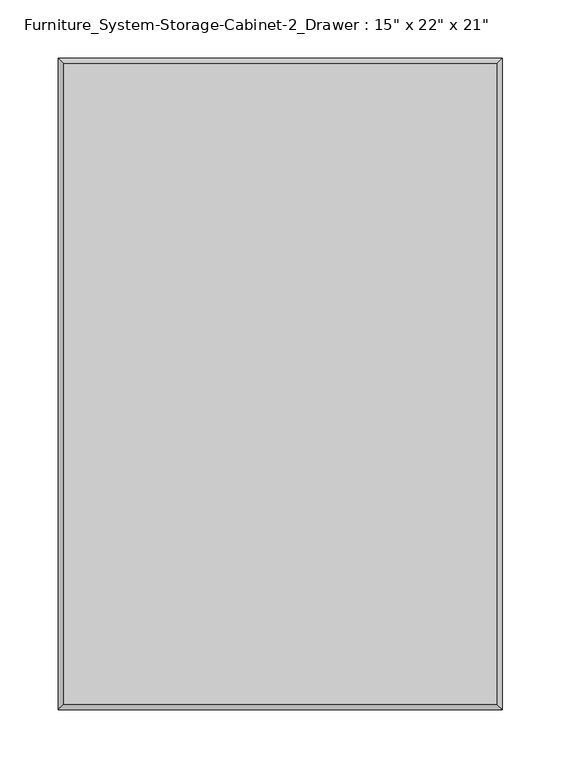
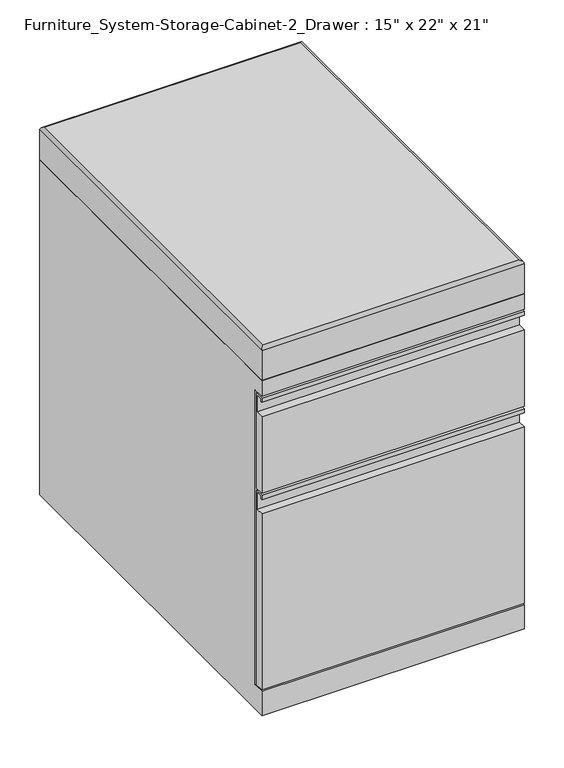
"""IFC4 building model written with IfcOpenShell, lengths in millimetres: furniture geometry."""

from ifc_helpers import new_model, si_unit, frame, origin, place, context, project, spatial, polyline, ellipse_curve, outline, extrude, source, transform, mapped, element, save
from ifc_brep_helpers import plane_surface, cylinder_surface, advanced_brep


def furniture_b20b6c06(model_context):
    return source(origin(), model_context, "Body", "SolidModel", [
        extrude(outline(polyline([(0.0, 360.3625), (0.0, 478.2451302), (11.8998876, 478.2451302), (11.8998876, 504.8884893), (1.5239879, 504.8884893), (1.5239879, 500.0625121), (0.0, 500.0625121), (0.0, 506.4124879), (13.4873883, 506.4124879), (13.4873883, 360.3625), (0.0, 360.3625)])), frame((-190.5, 0.0, 0.0), z_axis=(1.0, 0.0, 0.0), x_axis=(0.0, 1.0, 0.0)), (0.0, 0.0, 1.0), 381.0),
        extrude(outline(polyline([(0.0, 58.7374985), (0.0, 329.0201544), (11.9293774, 329.0201544), (11.9293774, 355.6635136), (1.5239879, 355.6635136), (1.5239879, 350.8375), (0.0, 350.8375), (0.0, 357.1875121), (13.4873883, 357.1875121), (13.4873883, 58.7374985), (0.0, 58.7374985)])), frame((-190.5, 0.0, 0.0), z_axis=(1.0, 0.0, 0.0), x_axis=(0.0, 1.0, 0.0)), (0.0, 0.0, 1.0), 381.0),
        extrude(outline(polyline([(56.820048, 9.2063177), (51.9174039, 19.05), (100.4825718, 19.05), (95.5799278, 9.2063177), (86.9277397, 2.4185626), (76.1999879, 0.0), (65.4722406, 2.4185626), (56.820048, 9.2063177)])), frame((-136.525, 0.0, 0.0), z_axis=(1.0, 0.0, 0.0), x_axis=(0.0, 1.0, 0.0)), (0.0, 0.0, 1.0), 44.45),
        extrude(outline(polyline([(463.2200601, 9.2063177), (458.317416, 19.05), (506.882584, 19.05), (501.9799399, 9.2063177), (493.3277518, 2.4185626), (482.6, 0.0), (471.8722527, 2.4185626), (463.2200601, 9.2063177)])), frame((-136.525, 0.0, 0.0), z_axis=(1.0, 0.0, 0.0), x_axis=(0.0, 1.0, 0.0)), (0.0, 0.0, 1.0), 44.45),
        extrude(outline(polyline([(56.820048, 9.2063177), (51.9174039, 19.05), (100.4825718, 19.05), (95.5799278, 9.2063177), (86.9277397, 2.4185626), (76.1999879, 0.0), (65.4722406, 2.4185626), (56.820048, 9.2063177)])), frame((92.075, 0.0, 0.0), z_axis=(1.0, 0.0, 0.0), x_axis=(0.0, 1.0, 0.0)), (0.0, 0.0, 1.0), 44.45),
        extrude(outline(polyline([(506.882584, 19.05), (501.9799399, 9.2063177), (493.3277518, 2.4185626), (482.6, 0.0), (471.8722527, 2.4185626), (463.2200601, 9.2063177), (458.317416, 19.05), (506.882584, 19.05)])), frame((92.075, 0.0, 0.0), z_axis=(1.0, 0.0, 0.0), x_axis=(0.0, 1.0, 0.0)), (0.0, 0.0, 1.0), 44.45),
        extrude(outline(polyline([(0.0, 533.4), (558.8, 533.4), (558.8, 19.05), (0.0, 19.05), (0.0, 56.3562485), (16.6623883, 56.3562485), (16.6623883, 509.5875121), (0.0, 509.5875121), (0.0, 533.4)])), frame((-190.5, 0.0, 0.0), z_axis=(1.0, 0.0, 0.0), x_axis=(0.0, 1.0, 0.0)), (0.0, 0.0, 1.0), 381.0),
        advanced_brep(
        [(185.7375, 4.7625, 584.2), (185.7375, 554.0375, 584.2), (-185.7375, 554.0375, 584.2), (-185.7375, 4.7625, 584.2), (190.5, 558.8, 533.4), (190.5, 0.0, 533.4), (-190.5, 0.0, 533.4), (-190.5, 558.8, 533.4), (-190.5, 558.8, 579.4375), (190.5, 558.8, 579.4375), (-190.5, 0.0, 579.4375), (190.5, 0.0, 579.4375)],
        [
            (0, 1),
            (1, 2),
            (2, 3),
            (3, 0),
            (4, 5),
            (5, 6),
            (6, 7),
            (7, 4),
            (7, 8),
            (8, 9),
            (9, 4),
            (6, 10),
            (10, 8),
            (5, 11),
            (11, 10),
            (9, 11),
            (0, 11, ellipse_curve(frame((185.7375, 4.7625, 579.4375), z_axis=(0.7071067811865475, 0.7071067811865475, 0.0), x_axis=(0.7071067811865474, -0.7071067811865476, 0.0)), 6.7351921, 4.7625)),
            (9, 1, ellipse_curve(frame((185.7375, 554.0375, 579.4375), z_axis=(0.7071067811865475, -0.7071067811865475, 0.0), x_axis=(-0.7071067811865474, -0.7071067811865476, 0.0)), 6.7351921, 4.7625)),
            (3, 10, ellipse_curve(frame((-185.7375, 4.7625, 579.4375), z_axis=(0.7071067811865475, -0.7071067811865475, 0.0), x_axis=(-0.7071067811865476, -0.7071067811865474, 0.0)), 6.7351921, 4.7625)),
            (2, 8, ellipse_curve(frame((-185.7375, 554.0375, 579.4375), z_axis=(-0.7071067811865475, -0.7071067811865475, 0.0), x_axis=(-0.7071067811865474, 0.7071067811865476, 0.0)), 6.7351921, 4.7625)),
        ],
        [
            plane_surface(frame((-190.5, 558.8, 584.2), z_axis=(0.0, 0.0, 1.0), x_axis=(-1.0, 0.0, 0.0))),
            plane_surface(frame((-190.5, 558.8, 533.4), z_axis=(0.0, 0.0, -1.0), x_axis=(1.0, 0.0, 0.0))),
            plane_surface(frame((190.5, 558.8, 584.2), z_axis=(0.0, 1.0, 0.0), x_axis=(0.0, 0.0, -1.0))),
            plane_surface(frame((-190.5, 558.8, 584.2), z_axis=(-1.0, 0.0, 0.0), x_axis=(0.0, 0.0, -1.0))),
            plane_surface(frame((-190.5, 0.0, 584.2), z_axis=(0.0, -1.0, 0.0), x_axis=(0.0, 0.0, -1.0))),
            plane_surface(frame((190.5, 0.0, 584.2), z_axis=(1.0, 0.0, 0.0), x_axis=(0.0, 0.0, -1.0))),
            cylinder_surface(frame((185.7375, 558.8, 579.4375), z_axis=(0.0, -1.0, 0.0), x_axis=(1.0, 0.0, 0.0)), 4.7625),
            cylinder_surface(frame((190.5, 4.7625, 579.4375), z_axis=(-1.0, 0.0, 0.0), x_axis=(0.0, -1.0, 0.0)), 4.7625),
            cylinder_surface(frame((-185.7375, 0.0, 579.4375), z_axis=(0.0, 1.0, 0.0), x_axis=(-1.0, 0.0, 0.0)), 4.7625),
            cylinder_surface(frame((-190.5, 554.0375, 579.4375), z_axis=(1.0, 0.0, 0.0), x_axis=(0.0, 1.0, 0.0)), 4.7625),
        ],
        [
            (0, [[1, 2, 3, 4]]),
            (1, [[5, 6, 7, 8]]),
            (2, [[-8, 9, 10, 11]]),
            (3, [[-7, 12, 13, -9]]),
            (4, [[-6, 14, 15, -12]]),
            (5, [[-5, -11, 16, -14]]),
            (6, [[17, -16, 18, -1]]),
            (7, [[-17, -4, 19, -15]]),
            (8, [[-19, -3, 20, -13]]),
            (9, [[-18, -10, -20, -2]]),
        ],
    ),
    ])


if __name__ == "__main__":
    model = new_model("IFC4")
    model_context = context("Model", 3, world=origin())
    ifc_project = project(units=[si_unit("LENGTHUNIT", "METRE", prefix="MILLI")], contexts=[model_context])
    site = spatial("IfcSite", under=ifc_project)
    building = spatial("IfcBuilding", under=site)
    placement = place(None, origin())
    furniture_shape = furniture_b20b6c06(model_context)
    element("IfcFurniture", 1, ObjectType="Furniture_System-Storage-Cabinet-2_Drawer : 15\" x 22\" x 21\"", at=placement, inside=building, context=model_context, shape_type="MappedRepresentation", body=[
        mapped(furniture_shape, transform((0.0, 0.0, 0.0), x_axis=(1.0, 0.0, 0.0), y_axis=(0.0, 1.0, 0.0), z_axis=(0.0, 0.0, 1.0))),
    ])
    save(model, "model.ifc")

# Revit data of these elements
# Type "Furniture_System-Storage-Cabinet-2_Drawer : 15\" x 22\" x 21\""
#   Type Comments = "15\" x 22\" x 21\" Double Drawer Cabinet"
#   Width = 1' - 3"
#   Height = 1' - 9"
#   Depth = 1' - 10"
#   Show Solid [instance default] = yes
#   Show Dashed [instance default] = no
#   Seat Visible [instance default] = yes
#   Drawer Material [instance default] = Metal - Paint - Beige
#   Cabinet Material [instance default] = Metal - Paint - Beige
#   Model = ""
#   Manufacturer = ""
#   Keynote = ""
#   Description = (empty or 0)
#   Default Elevation = 0
# Element 1 (IfcFurniture, "Furniture_System-Storage-Cabinet-2_Drawer : 15\" x 22\" x 21\"")
#   Materials on its faces: "Metal - Paint - Beige"
# Materials
#   "Metal - Paint - Beige": class "Metal", colour RGB 247 225 182, transparency 0
